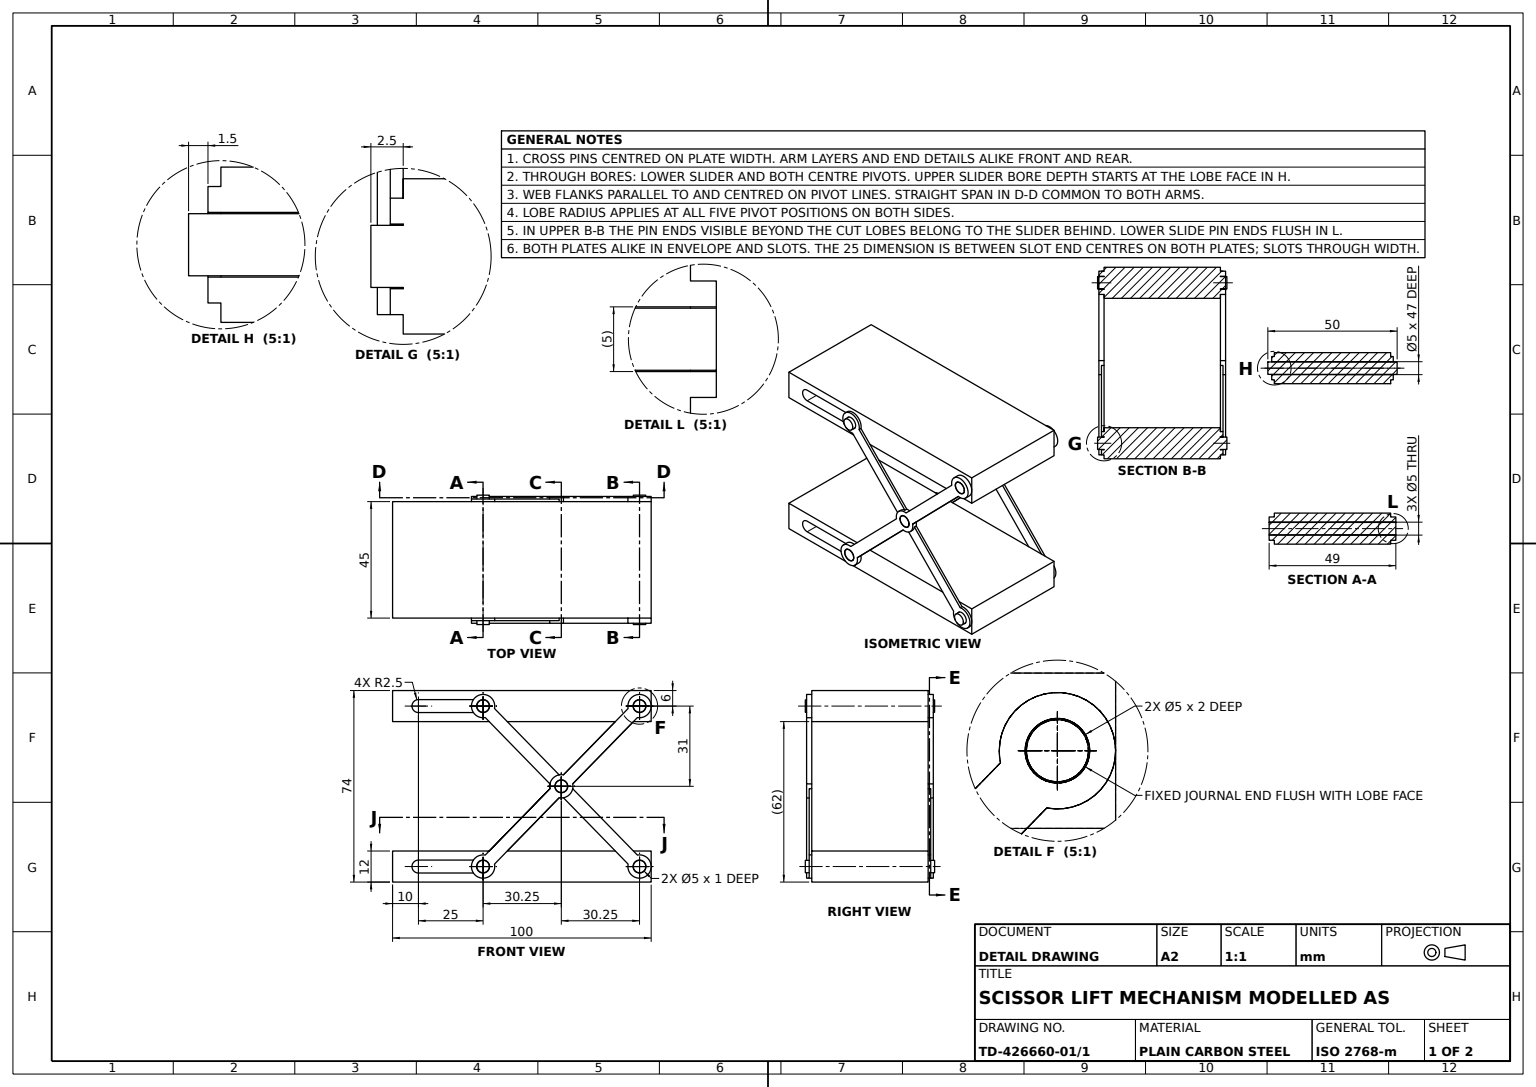
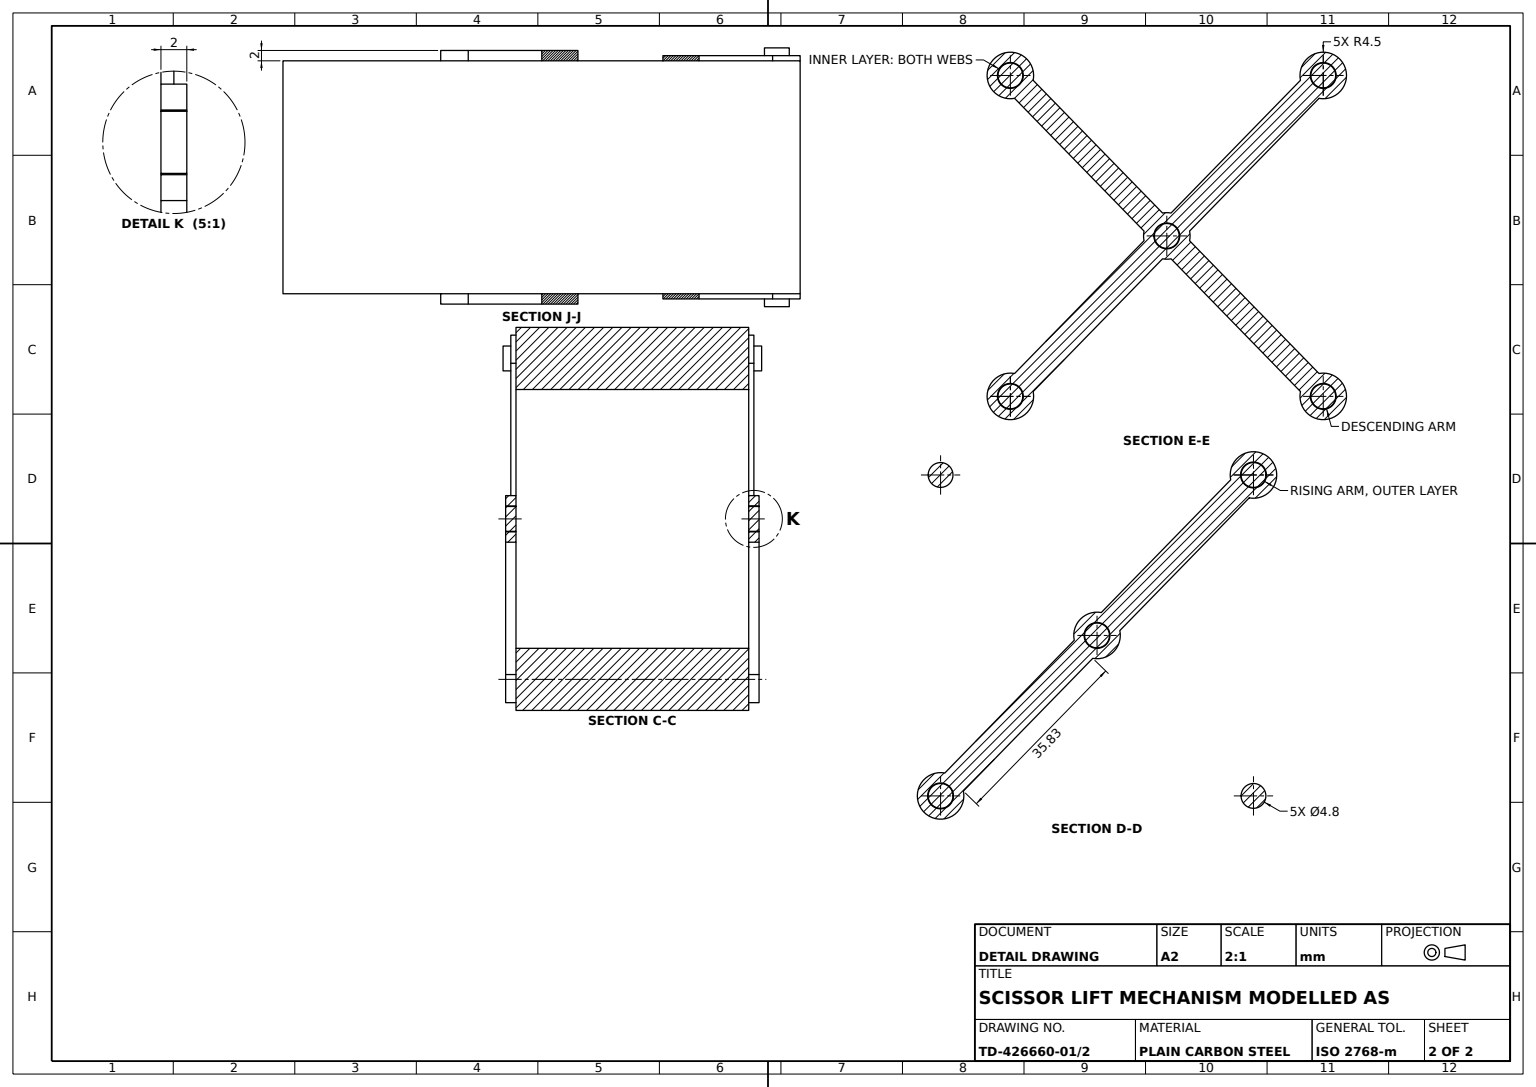
SolidWorks part; units mm, degrees
material "Plain Carbon Steel"
ref_plane "Front Plane" through (0, 0, 0) normal (0, 0, 1) x (1, 0, 0)
ref_plane "Top Plane" through (0, 0, 0) normal (0, 1, 0) x (1, 0, 0)
ref_plane "Right Plane" through (0, 0, 0) normal (1, 0, 0) x (0, 0, -1)
sketch "Base Plate Sketch" plane through (0, 0, 0) normal (0, 1, 0) x (1, 0, 0)
  line L1 (-50, 22.5) -> (50, 22.5)
  line L2 (-50, 22.5) -> (-50, -22.5)
  line L3 (-50, -22.5) -> (50, -22.5)
  line L4 (50, 22.5) -> (50, -22.5)
  line L5 (-50, 22.5) -> (50, -22.5) construction
  line L6 (-50, -22.5) -> (50, 22.5) construction
  point P0 (0, 0)
  dimension "D1" = 45
  dimension "D2" = 100
extrude "Base Plate" add sketch "Base Plate Sketch" along normal blind 12
sketch "Base Plate Guide Slot Sketch" plane through (0, 0, 22.5) normal (0, 0, 1) x (1, 0, 0)
  line L0 (-50, 12) -> (50, 12) construction
  line L2 (-15, 6) -> (-40, 6) construction
  line L3 (50, 12) -> (50, 0) construction
  line L4 (-15, 3.5) -> (-40, 3.5)
  line L5 (-15, 8.5) -> (-40, 8.5)
  arc A0 (-15, 3.5) -> (-15, 8.5) centre (-15, 6) ccw
  arc A1 (-40, 8.5) -> (-40, 3.5) centre (-40, 6) ccw
  point P9 (-27.5, 6)
  dimension "D2" = 25
  dimension "D1" = 5
  dimension "D3" = 6
  dimension "D4" = 65
extrude "Base Plate Guide Slot" cut sketch "Base Plate Guide Slot Sketch" against normal blind 200
ref_plane "Plane1" through (0, 62, 0) normal (0, 1, 0) x (1, 0, 0)
sketch "Top Plate Sketch" plane through (0, 62, 0) normal (0, 1, 0) x (1, 0, 0)
  line L1 (-50, 22.5) -> (50, 22.5)
  line L2 (-50, 22.5) -> (-50, -22.5)
  line L3 (-50, -22.5) -> (50, -22.5)
  line L4 (50, 22.5) -> (50, -22.5)
  line L5 (-50, 22.5) -> (50, -22.5) construction
  line L6 (-50, -22.5) -> (50, 22.5) construction
  point P0 (0, 0)
extrude "Top Plate" add sketch "Top Plate Sketch" along normal blind 12 separate body
sketch "Top Plate Guide Slot Sketch" plane through (0, 0, 22.5) normal (0, 0, 1) x (1, 0, 0)
  line L0 (-15, 68) -> (-40, 68) construction
  line L1 (-50, 74) -> (50, 74) construction
  line L2 (-15, 65.5) -> (-40, 65.5)
  line L3 (-15, 70.5) -> (-40, 70.5)
  line L4 (50, 74) -> (50, 62) construction
  arc A0 (-15, 65.5) -> (-15, 70.5) centre (-15, 68) ccw
  arc A1 (-40, 70.5) -> (-40, 65.5) centre (-40, 68) ccw
  point P4 (-27.5, 68)
  dimension "D3" = 2.5
  dimension "D1" = 6
  dimension "D2" = 65
  dimension "D4" = 25
extrude "Top Plate Guide Slot" cut sketch "Top Plate Guide Slot Sketch" against normal blind 50
sketch "Front Scissor Arm A Sketch" plane through (0, 0, 22.5) normal (0, 0, 1) x (1, 0, 0)
  line L1 (50, 12) -> (50, 0) construction
  line L2 (-50, 12) -> (50, 12) construction
  line L4 (-14.1761, 63.5761) -> (10.8476, 37.932)
  line L5 (-10.5976, 67.068) -> (14.4261, 41.4239)
  line L7 (19.6524, 36.068) -> (44.6761, 10.4239)
  line L10 (16.0739, 32.5761) -> (41.0976, 6.932)
  line L13 (-50, 0) -> (50, 0) construction
  circle A0 centre (-15, 68) radius 2.5
  circle A1 centre (45.5, 6) radius 2.5
  arc A2 (-10.5976, 67.068) -> (-14.1761, 63.5761) centre (-15, 68) ccw
  arc A3 (41.0976, 6.932) -> (44.6761, 10.4239) centre (45.5, 6) ccw
  circle A8 centre (15.25, 37) radius 2.5
  arc A11 (10.8476, 37.932) -> (16.0739, 32.5761) centre (15.25, 37) ccw
  arc A12 (19.6524, 36.068) -> (14.4261, 41.4239) centre (15.25, 37) ccw
  point P13 (0, 0)
  dimension "D1" = 5
  dimension "D2" = 5
  dimension "D3" = 9
  dimension "D4" = 9
  dimension "D7" = 9
  dimension "D8" = 15.25
  dimension "D9" = 35.8302
  dimension "D10" = 55.2737
  dimension "D16" = 5
  dimension "D5" = 4.5
  dimension "D6" = 6
  dimension "D11" = 79.1438
  dimension "D20" = 25
  dimension "D21" = 35.8302
extrude "Front Scissor Arm A" add sketch "Front Scissor Arm A Sketch" along normal blind 1
sketch "Front Scissor Arm B Sketch" plane through (0, 0, 22.5) normal (0, 0, 1) x (1, 0, 0)
  line L0 (50, 74) -> (50, 62) construction
  line L1 (-50, 74) -> (50, 74) construction
  line L2 (16.0739, 41.4239) -> (41.0976, 67.068)
  line L3 (-10.5976, 6.932) -> (14.4261, 32.5761)
  line L4 (-14.1761, 10.4239) -> (10.8476, 36.068)
  line L5 (19.6524, 37.932) -> (44.6761, 63.5761)
  circle A0 centre (-15, 6) radius 2.5
  arc A1 (-14.1761, 10.4239) -> (-10.5976, 6.932) centre (-15, 6) ccw
  circle A2 centre (45.5, 68) radius 2.5
  arc A3 (44.6761, 63.5761) -> (41.0976, 67.068) centre (45.5, 68) ccw
  circle A4 centre (15.25, 37) radius 2.5
  arc A5 (14.4261, 32.5761) -> (19.6524, 37.932) centre (15.25, 37) ccw
  arc A6 (16.0739, 41.4239) -> (10.8476, 36.068) centre (15.25, 37) ccw
  dimension "D1" = 9
  dimension "D2" = 5
  dimension "D5" = 9
  dimension "D6" = 5
  dimension "D9" = 9
  dimension "D3" = 4.5
  dimension "D4" = 6
  dimension "D7" = 15.25
  dimension "D8" = 79.1438
  dimension "D10" = 79.1438
  dimension "D11" = 43.3135
  dimension "D12" = 25.0237
  dimension "D13" = 25.6441
extrude "Front Scissor Arm B" add sketch "Front Scissor Arm B Sketch" along normal blind 2
sketch "Front Arm Link Pin Sketch" plane through (0, 0, 24.5) normal (0, 0, 1) x (1, 0, 0)
  circle A0 centre (15.25, 37) radius 2.5
  circle A1 centre (15.25, 37) radius 4.5
  dimension "D1" = 9
  dimension "D2" = 5
extrude "Front Arm Link Pin" add sketch "Front Arm Link Pin Sketch" against normal blind 2
sketch "Center Pivot Pin Front Sketch" plane through (0, 0, 24.5) normal (0, 0, 1) x (1, 0, 0)
  circle A0 centre (15.25, 37) radius 2.4
  dimension "D1" = 4.8
extrude "Center Pivot Pin Front Ø4.8" add sketch "Center Pivot Pin Front Sketch" against normal blind 2 separate body
sketch "Lower Cross Pin Sketch" plane through (0, 0, 24.5) normal (0, 0, 1) x (1, 0, 0)
  circle A0 centre (-15, 6) radius 2.4
  dimension "D1" = 4.8
extrude "Lower Cross Pin Ø4.8x49" add sketch "Lower Cross Pin Sketch" against normal blind 49 separate body
sketch "Upper Cross Pin Head Sketch" plane through (0, 0, 23.5) normal (0, 0, 1) x (1, 0, 0)
  circle A0 centre (-15, 68) radius 2.4
  dimension "D1" = 4.8
extrude "Upper Cross Pin Head" add sketch "Upper Cross Pin Head Sketch" along normal blind 1.5 separate body
sketch "Upper Cross Pin Sketch" plane through (0, 0, 25) normal (0, 0, 1) x (1, 0, 0)
  circle A0 centre (-15, 68) radius 2.4
  dimension "D1" = 4.8
extrude "Upper Cross Pin Ø4.8x47.5" add sketch "Upper Cross Pin Sketch" against normal blind 47.5
sketch "Front Arm Pin Sketch" plane through (0, 0, 22.5) normal (0, 0, 1) x (1, 0, 0)
  circle A0 centre (45.5, 68) radius 2.4
  dimension "D1" = 4.8
extrude "Front Arm Pin Ø4.8" add sketch "Front Arm Pin Sketch" along normal blind 2
sketch "Lower Roller Pin Sketch" plane through (0, 0, 22.5) normal (0, 0, 1) x (1, 0, 0)
  circle A0 centre (45.5, 6) radius 2.4
  dimension "D1" = 4.8
extrude "Lower Roller Pin Ø4.8" add sketch "Lower Roller Pin Sketch" along normal blind 2.5
sketch "Rear Scissor Arm A Sketch" plane through (0, 0, -22.5) normal (0, 0, -1) x (-1, 0, 0)
  line L0 (-50, 12) -> (-50, 0) construction
  line L1 (-50, 12) -> (50, 12) construction
  line L2 (-14.4261, 41.4239) -> (10.5976, 67.068)
  line L3 (-41.0976, 6.932) -> (-16.0739, 32.5761)
  line L4 (-44.6761, 10.4239) -> (-19.6524, 36.068)
  line L5 (-10.8476, 37.932) -> (14.1761, 63.5761)
  circle A0 centre (15, 68) radius 2.5
  arc A1 (14.1761, 63.5761) -> (10.5976, 67.068) centre (15, 68) ccw
  circle A2 centre (-45.5, 6) radius 2.5
  arc A3 (-44.6761, 10.4239) -> (-41.0976, 6.932) centre (-45.5, 6) ccw
  arc A4 (-16.0739, 32.5761) -> (-10.8476, 37.932) centre (-15.25, 37) ccw
  circle A5 centre (-15.25, 37) radius 2.5
  arc A6 (-14.4261, 41.4239) -> (-19.6524, 36.068) centre (-15.25, 37) ccw
  dimension "D1" = 4.5
  dimension "D3" = 9
  dimension "D4" = 5
  dimension "D5" = 9
  dimension "D6" = 5
  dimension "D9" = 9
  dimension "D10" = 5
  dimension "D2" = 6
  dimension "D7" = 79.1438
  dimension "D8" = 56.6441
  dimension "D11" = 56.6441
  dimension "D12" = 55.2737
  dimension "D13" = 30.25
  dimension "D14" = 37
extrude "Rear Scissor Arm A" add sketch "Rear Scissor Arm A Sketch" along normal blind 1
sketch "Upper Cross Pin End Sketch" plane through (0, 0, -22.5) normal (0, 0, -1) x (-1, 0, 0)
  circle A0 centre (15, 68) radius 2.4
  circle A1 centre (-45.5, 6) radius 2.4
  dimension "D1" = 4.8
  dimension "D2" = 4.8
extrude "Upper Cross Pin End Ø4.8" add sketch "Upper Cross Pin End Sketch" along normal blind 2.5
sketch "Rear Scissor Arm B Sketch" plane through (0, 0, -22.5) normal (0, 0, -1) x (-1, 0, 0)
  line L0 (-50, 74) -> (50, 74) construction
  line L1 (-50, 74) -> (-50, 62) construction
  line L2 (-10.8476, 36.068) -> (14.1761, 10.4239)
  line L3 (-44.6761, 63.5761) -> (-19.6524, 37.932)
  line L4 (-41.0976, 67.068) -> (-16.0739, 41.4239)
  line L5 (-14.4261, 32.5761) -> (10.5976, 6.932)
  line L6 (18.7417, 70.5) -> (40, 70.5) construction
  circle A0 centre (-45.5, 68) radius 2.5
  arc A1 (-41.0976, 67.068) -> (-44.6761, 63.5761) centre (-45.5, 68) ccw
  circle A2 centre (15, 6) radius 2.5
  arc A3 (10.5976, 6.932) -> (14.1761, 10.4239) centre (15, 6) ccw
  circle A4 centre (-15.25, 37) radius 2.5
  arc A5 (-19.6524, 37.932) -> (-14.4261, 32.5761) centre (-15.25, 37) ccw
  arc A6 (-10.8476, 36.068) -> (-16.0739, 41.4239) centre (-15.25, 37) ccw
  point P11 (-47.2893, 66.254)
  point P12 (13.2107, 4.254)
  dimension "D1" = 9
  dimension "D2" = 5
  dimension "D3" = 9
  dimension "D4" = 5
  dimension "D7" = 9
  dimension "D8" = 5
  dimension "D5" = 6
  dimension "D6" = 4.5
  dimension "D9" = 4.9454
  dimension "D10" = 8.524
  dimension "D11" = 9.3479
  dimension "D12" = 16.4997
  dimension "D13" = 20.0783
  dimension "D14" = 20.9021
  dimension "D15" = 21.726
  dimension "D16" = 25.3046
  dimension "D17" = 46.7497
  dimension "D18" = 50.3283
  dimension "D19" = 29.0761
  dimension "D20" = 60.0761
extrude "Rear Scissor Arm B" add sketch "Rear Scissor Arm B Sketch" along normal blind 2
sketch "Center Pivot Pin Rear Sketch" plane through (0, 0, -24.5) normal (0, 0, -1) x (-1, 0, 0)
  circle A0 centre (-15.25, 37) radius 2.4
  dimension "D1" = 4.8
extrude "Center Pivot Pin Rear Ø4.8" add sketch "Center Pivot Pin Rear Sketch" against normal blind 2 separate body
sketch "Rear Arm Pin Sketch" plane through (0, 0, -22.5) normal (0, 0, -1) x (-1, 0, 0)
  circle A0 centre (-45.5, 68) radius 2.4
  dimension "D1" = 4.8
extrude "Rear Arm Pin Ø4.8" add sketch "Rear Arm Pin Sketch" along normal blind 2
